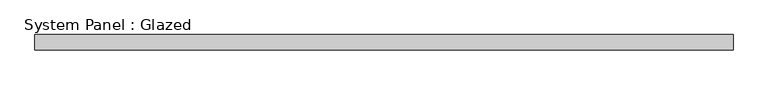
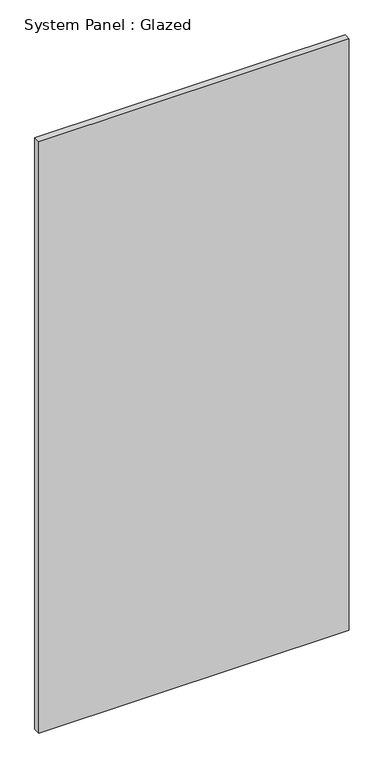
"""IFC4 building model written with IfcOpenShell, lengths in millimetres: plate geometry, System Panel : Glazed."""

from ifc_helpers import new_model, si_unit, origin, origin_with_axes, place, context, project, spatial, polyline, outline, extrude, source, transform, mapped, element, save


def system_panel_glazed_3d427df9(model_context):
    return source(origin(), model_context, "Body", "SweptSolid", [
        extrude(outline(polyline([(582.0833333, 19.05), (-582.0833333, 19.05), (-582.0833333, 44.45), (582.0833333, 44.45), (582.0833333, 19.05)])), origin_with_axes(), (0.0, 0.0, 1.0), 2343.15),
    ])


if __name__ == "__main__":
    model = new_model("IFC4")
    model_context = context("Model", 3, world=origin())
    ifc_project = project(units=[si_unit("LENGTHUNIT", "METRE", prefix="MILLI")], contexts=[model_context])
    site = spatial("IfcSite", under=ifc_project)
    building = spatial("IfcBuilding", under=site)
    placement = place(None, origin())
    system_panel_glazed_shape = system_panel_glazed_3d427df9(model_context)
    element("IfcPlate", 1, ObjectType="System Panel : Glazed", at=placement, inside=building, context=model_context, shape_type="MappedRepresentation", body=[
        mapped(system_panel_glazed_shape, transform((0.0, 0.0, 0.0), x_axis=(1.0, 0.0, 0.0), y_axis=(0.0, 1.0, 0.0), z_axis=(0.0, 0.0, 1.0))),
    ])
    save(model, "model.ifc")

# Revit data of these elements
# Type "System Panel : Glazed"
#   Construction Type Id = "GSP4R"
#   Analytic Construction = "1/8 in Pilkington single glazing"
#   Visual Light Transmittance = 0.9
#   Solar Heat Gain Coefficient = 0.86
#   Heat Transfer Coefficient (U) = 1.18115 BTU/(h·ft²·°F)
# Element 1 (IfcPlate, "System Panel : Glazed")
#   Materials on its faces: "Glass"
# Materials
#   "Glass": class "Glass", colour RGB 0 128 192, transparency 0.75, Description = "Soda Lime Glass", Cost = 0
